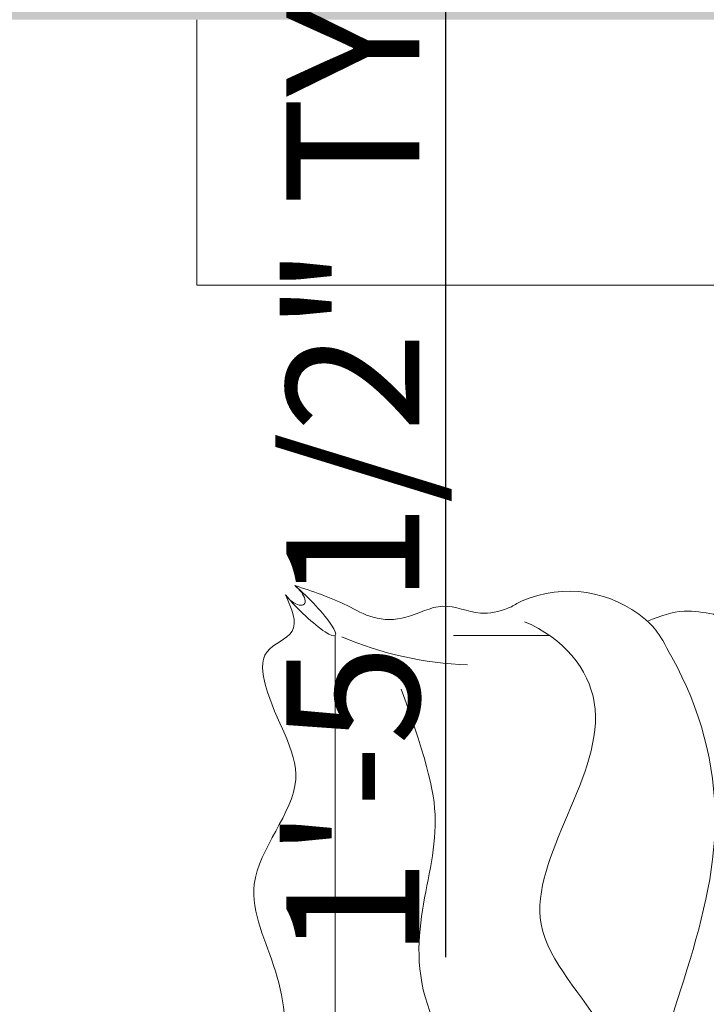
# Model space of a CAD drawing. Units: inches. Extents: x 2083 to 3317, y 1141 to 2115.
# Tile 122 of 256: x 3006 to 3068, y 1327 to 1416. Entities that reach past the tile are written whole.
import ezdxf

# ---------------------------------------------------------------- set-up
doc = ezdxf.new("R2010")
doc.units = ezdxf.units.IN
for name, color, linetype, lineweight in [('A-ANNO-DIMS', 2, 'Continuous', 18), ('A-FLOR-CASE', 8, 'Continuous', 18), ('A-FURN', 8, 'Continuous', 18), ('www.cadblocksfree.com', 7, 'Continuous', 9)]:
    doc.layers.add(name, color=color, linetype=linetype, lineweight=lineweight)
doc.layers.add('A-WALL-PATT', color=251, linetype='Continuous', lineweight=13, true_color=0x636466)
doc.styles.get("Standard").update_dxf_attribs({"font": 'arial.ttf'})
doc.dimstyles.new('ISO-25', dxfattribs={"dimtxt": 12, "dimasz": 12, "dimexe": 1.25, "dimexo": 0.625, "dimtad": 1, "dimlunit": 3, "dimtxsty": 'Standard', "dimcen": 2.5, "dimadec": 0, "dimazin": 0, "dimtfac": 1, "dimtmove": 0, "dimatfit": 3, "dimfxl": 1, "dimarcsym": 0})

# ---------------------------------------------------------------- blocks, each defined once
blk = doc.blocks.new('bed')
at = {"layer": 'www.cadblocksfree.com', "ltscale": 0.2}
for p, q in [((3363.387, 1412.3), (3363.387, 1402.937)), ((3363.387, 1391.414), (3426.379, 1391.414))]:
    blk.add_line(p, q, dxfattribs=at)
for centre, radius, start, end in [((3370.55, 1414.186), 11.465, 139.46484, 203.37116), ((3367.278, 1412.869), 7.939, 204.0179, 212.61896), ((3331.909, 1405.558), 34.378, 336.84952, 357.90025)]:
    blk.add_arc(centre, radius, start, end, dxfattribs=at)
at = {"layer": 'www.cadblocksfree.com', "ltscale": 0.2, "extrusion": (0, 0, -1)}
for centre, major_axis, ratio, start_param, end_param in [((3360.344, 1388.371), (3.043, 3.043), 0.168252, 4.250342, 8.316029), ((3359.289, 1387.316), (1.055, 1.055), 0.453532, 4.422107, 8.144264)]:
    blk.add_ellipse(centre, major_axis=major_axis, ratio=ratio, start_param=start_param, end_param=end_param, dxfattribs=at)
at = {"layer": 'www.cadblocksfree.com', "ltscale": 0.2}
for points, knots in [([(3365.512, 1424.213), (3370.519, 1427.004), (3381.149, 1429.825), (3396.214, 1425.866), (3410.541, 1420.654), (3420.273, 1432.695), (3425.882, 1426.771), (3428.534, 1423.97)], [0.099185, 0.099185, 0.099185, 0.099185, 0.523647, 0.927087, 1.289918, 1.564439, 1.810555, 1.810555, 1.810555, 1.810555]), ([(3361.336, 1428.309), (3361.334, 1428.297), (3361.16, 1427.338), (3360.778, 1425.173), (3361.469, 1423.14), (3362.014, 1421.845)], [0.3128349, 0.3128349, 0.3128349, 0.3128349, 0.313751, 0.386958, 0.4759027, 0.4759027, 0.4759027, 0.4759027]), ([(3362.057, 1409.866), (3363.638, 1413.65), (3372.978, 1421.337), (3389.682, 1406.045), (3402.396, 1419.984), (3416.037, 1420.167), (3423.233, 1415.231), (3427.827, 1408.899)], [0.029901, 0.029901, 0.029901, 0.029901, 0.276967, 0.797115, 1.093669, 1.464666, 1.788489, 1.788489, 1.788489, 1.788489]), ([(3358.529, 1387.473), (3359.098, 1389.205), (3359.955, 1391.816), (3361.924, 1395.149), (3361.896, 1398.555), (3359.883, 1401.841), (3361.557, 1405.208), (3361.034, 1407.507), (3360.643, 1408.467), (3360.591, 1408.59)], [0, 0, 0, 0, 0.138875, 0.2092702, 0.2901949, 0.3858479, 0.4804923, 0.5489252, 0.5590752, 0.5590752, 0.5590752, 0.5590752]), ([(3368.632, 1397.839), (3375.978, 1400.489), (3385.349, 1402.757), (3397.531, 1395.273), (3413.593, 1410.377), (3407.806, 1395.019), (3420.759, 1398.2)], [0.029901, 0.029901, 0.029901, 0.029901, 0.276967, 0.797115, 1.093669, 1.16836, 1.16836, 1.16836, 1.16836]), ([(3430.32, 1386.556), (3427.327, 1387.653), (3422.148, 1389.55), (3414.529, 1384.137), (3405.607, 1387.046), (3396.29, 1386.314), (3386.838, 1381.282), (3377.742, 1390.272), (3370.778, 1384.799), (3364.626, 1383.966), (3363.275, 1388.265), (3360.778, 1387.151), (3359.446, 1386.556)], [0, 0, 0, 0, 8.93042, 15.449194, 25.485629, 34.878505, 43.598887, 54.554403, 64.16647, 67.461673, 70.610457, 74.213583, 74.213583, 74.213583, 74.213583])]:
    blk.add_open_spline(points, degree=3, knots=knots, dxfattribs=at)
for points in [[(3361.235, 1424.042), (3361.236, 1424.042), (3361.237, 1424.043), (3361.239, 1424.043)], [(3361.837, 1421.637), (3362.352, 1422.25), (3362.867, 1422.863), (3365.512, 1424.213)]]:
    blk.add_open_spline(points, degree=3, dxfattribs=at)
blk = doc.blocks.new('CASEWORK-96X24')
for q in [(0, 0), (24, 96)]:
    blk.add_line((0, 96), q)
blk = doc.blocks.new('*D19')
at = {"layer": 'A-ANNO-DIMS', "color": 0, "lineweight": -2, "transparency": 16777216}
for p, q in [((3044.457, 1486.497), (3044.457, 1498.497)), ((3041.693, 1474.497), (3045.707, 1474.497)), ((3044.457, 1474.497), (3044.457, 1456.781)), ((3041.693, 1456.781), (3045.707, 1456.781)), ((3044.457, 1444.781), (3044.457, 1331.553))]:
    blk.add_line(p, q, dxfattribs=at)
at = {"layer": 'A-ANNO-DIMS', "color": 0, "transparency": 16777216}
for points in [[(3042.457, 1486.497), (3046.457, 1486.497), (3044.457, 1474.497)], [(3042.457, 1444.781), (3046.457, 1444.781), (3044.457, 1456.781)]]:
    blk.add_solid(points, dxfattribs=at)
at = {"layer": 'Defpoints', "color": 0, "transparency": 16777216}
for p in [(3041.068, 1474.497), (3041.068, 1456.781), (3044.457, 1456.781)]:
    blk.add_point(p, dxfattribs=at)
at = {"layer": 'A-ANNO-DIMS', "color": 0, "transparency": 16777216, "insert": (3037.627, 1382.167), "char_height": 12, "attachment_point": 5, "rotation": 90}
blk.add_mtext('1\'-5 1/2" TYP.', dxfattribs=at)

msp = doc.modelspace()

# ---------------------------------------------------------------- hatches: boundary and pattern name
at = {"layer": 'A-WALL-PATT'}
h = msp.add_hatch(color=256, dxfattribs=at)
h.dxf.hatch_style = 1
h.paths.add_polyline_path([(3126.96, 2020.761), (2748.96, 2020.761), (2604.96, 2020.761), (2226.96, 2020.761), (2226.96, 1702.761), (2466.96, 1702.761), (2466.96, 1582.761), (2418.96, 1582.761), (2418.96, 1477.761), (2226.96, 1477.761), (2226.96, 1263.261), (2544.96, 1263.261), (2544.96, 1411.761), (2604.96, 1411.761), (2685.96, 1411.761), (2685.96, 1420.761), (2604.96, 1420.761), (2604.96, 1573.761), (2604.96, 1702.761), (2604.96, 2011.761), (2748.96, 2011.761), (2748.96, 1702.761), (2862.96, 1702.761), (2862.96, 1621.761), (2871.96, 1621.761), (2871.96, 1702.761), (2883.96, 1702.761), (2883.96, 1706.939, -0.026459), (2883.96, 1711.761), (2757.96, 1711.761), (2757.96, 1807.761), (2787.96, 1807.761), (2787.96, 1812.261), (2757.96, 1812.261), (2757.96, 2011.761), (2877.96, 2011.761), (2877.96, 1812.261), (2847.96, 1812.261), (2847.96, 1807.761), (2889.836, 1807.761), (2889.836, 1812.261), (2882.46, 1812.261), (2882.46, 2011.761), (3117.96, 2011.761), (3117.96, 1812.261), (2937.836, 1812.261), (2937.836, 1807.761), (2995.71, 1807.761), (2995.71, 1796.118), (3000.21, 1796.118), (3000.21, 1807.761), (3117.96, 1807.761), (3117.96, 1711.761), (3000.21, 1711.761), (3000.21, 1760.118), (2998.573, 1760.118, -0.020711), (2995.71, 1760.118), (2995.71, 1711.761), (2931.96, 1711.761), (2931.96, 1702.761), (3126.96, 1702.761)])
h.paths.add_polyline_path([(2471.46, 2011.761), (2471.46, 1810.011), (2462.717, 1810.011), (2462.717, 1805.511), (2505.96, 1805.511), (2505.96, 1810.011), (2475.96, 1810.011), (2475.96, 2011.761), (2595.96, 2011.761), (2595.96, 1810.011), (2565.96, 1810.011), (2565.96, 1805.511), (2595.96, 1805.511), (2595.96, 1711.761), (2235.96, 1711.761), (2235.96, 1805.511), (2353.71, 1805.511), (2353.71, 1796.054), (2358.21, 1796.054), (2358.21, 1805.511), (2414.717, 1805.511), (2414.717, 1810.011), (2235.96, 1810.011), (2235.96, 2011.761)], flags=16)
h.paths.add_polyline_path([(2270.205, 1994.61), (2270.205, 1970.61), (2246.205, 1970.61), (2246.205, 1994.61)], flags=0)
edge = h.paths.add_edge_path(flags=0)
edge.add_ellipse((2332.027, 1899.798), major_axis=(-3.043, 3.043), ratio=0.168252, start_angle=-161.33217, end_angle=-156.30711, ccw=False)
edge.add_ellipse((2333.082, 1898.744), major_axis=(-1.055, 1.055), ratio=0.453532, start_angle=-123.37102, end_angle=-94.15911)
edge = h.paths.add_edge_path(flags=0)
edge.add_ellipse((2332.027, 1968.876), major_axis=(3.043, 3.043), ratio=0.168252, start_angle=18.66783, end_angle=23.69289)
edge.add_spline(control_points=[(2332.926, 1970.691), (2332.227, 1970.336), (2330.894, 1969.659), (2328.413, 1970.932), (2327.204, 1967.749), (2324.71, 1969.956), (2322.533, 1967.012), (2320.013, 1971.296), (2317.68, 1968.158), (2316.041, 1967.102), (2315.427, 1966.81)], knot_values=[0, 0, 0, 0, 2.267059, 4.324559, 6.685584, 8.878641, 11.121502, 14.300359, 17.755284, 19.732645, 19.732645, 19.732645, 19.732645], degree=3, periodic=0)
edge.add_ellipse((2332.027, 1968.876), major_axis=(3.043, 3.043), ratio=0.168252, start_angle=18.66783, end_angle=23.69289, ccw=False)
edge.add_ellipse((2333.082, 1969.931), major_axis=(1.055, 1.055), ratio=0.453532, start_angle=56.62898, end_angle=85.84089, ccw=False)
edge = h.paths.add_edge_path(flags=0)
edge.add_spline(control_points=[(2296.428, 1967.988), (2293.628, 1965.336), (2287.704, 1959.727), (2299.744, 1949.996), (2294.533, 1935.669), (2290.573, 1920.604), (2293.394, 1909.974), (2296.185, 1904.967)], knot_values=[0.099185, 0.099185, 0.099185, 0.099185, 0.345301, 0.619822, 0.982653, 1.386093, 1.810555, 1.810555, 1.810555, 1.810555], degree=3, periodic=0)
edge.add_spline(control_points=[(2296.185, 1904.967), (2297.384, 1902.619), (2298.001, 1901.949), (2298.553, 1901.468)], knot_values=[0.006246, 0.006246, 0.006246, 0.006246, 0.055476, 0.055476, 0.055476, 0.055476], degree=3, periodic=0)
edge.add_spline(control_points=[(2298.553, 1901.468), (2297.259, 1900.923), (2295.225, 1900.232), (2293.06, 1900.614), (2292.101, 1900.788), (2292.09, 1900.791)], knot_values=[0.312835, 0.312835, 0.312835, 0.312835, 0.40178, 0.474987, 0.475903, 0.475903, 0.475903, 0.475903], degree=3, periodic=0)
edge.add_arc((2292.794, 1904.664), 3.937, 215.4209, 259.69818, ccw=False)
edge.add_spline(control_points=[(2289.585, 1902.382), (2289.477, 1902.535), (2289.368, 1902.688), (2289.261, 1902.841)], knot_values=[0.102872, 0.102872, 0.102872, 0.102872, 0.116896, 0.116896, 0.116896, 0.116896], degree=3, periodic=0)
edge.add_spline(control_points=[(2289.261, 1902.841), (2288.687, 1902.55), (2287.64, 1902.02), (2285.881, 1901.874), (2283.853, 1901.504), (2281.72, 1899.711), (2278.467, 1899.493), (2276.157, 1901.883), (2272.259, 1899.804), (2267.778, 1901.843), (2262.244, 1900.184), (2257.415, 1901.782), (2254.318, 1900.726), (2253.178, 1900.337)], knot_values=[0, 0, 0, 0, 1.907977, 3.477176, 5.261074, 7.972851, 11.680248, 13.717921, 16.939592, 22.789562, 27.502503, 33.595215, 37.145618, 37.145618, 37.145618, 37.145618], degree=3, periodic=0)
edge.add_line((2253.178, 1900.337), (2250.244, 1902.841))
edge.add_line((2250.244, 1902.841), (2250.244, 1965.833))
edge.add_line((2250.244, 1965.833), (2253.178, 1968.337))
edge.add_spline(control_points=[(2253.178, 1968.337), (2254.318, 1967.948), (2257.415, 1966.892), (2262.244, 1968.49), (2267.778, 1966.831), (2271.527, 1968.537), (2273.876, 1967.828), (2274.207, 1967.728)], knot_values=[0, 0, 0, 0, 0.09018, 0.244935, 0.364644, 0.513233, 0.537855, 0.537855, 0.537855, 0.537855], degree=3, periodic=0)
edge.add_arc((2274.353, 1963.793), 3.937, 72.05113, 92.12795, ccw=False)
edge.add_arc((2281.297, 1985.23), 18.596, 252.05113, 288.56572)
edge.add_arc((2292.317, 1956.029), 12.646, 71.02679, 113.77822, ccw=False)
edge = h.paths.add_edge_path(flags=0)
edge.add_spline(control_points=[(2274.899, 1951.856), (2275.066, 1951.617), (2275.233, 1951.377), (2275.398, 1951.136)], knot_values=[1.409916, 1.409916, 1.409916, 1.409916, 1.43159, 1.43159, 1.43159, 1.43159], degree=3, periodic=0)
edge.add_spline(control_points=[(2275.398, 1951.136), (2275.792, 1950.562), (2276.179, 1949.984), (2276.546, 1949.397)], knot_values=[1.358238, 1.358238, 1.358238, 1.358238, 1.409916, 1.409916, 1.409916, 1.409916], degree=3, periodic=0)
edge.add_line((2276.546, 1949.397), (2277.437, 1947.862))
edge.add_spline(control_points=[(2277.437, 1947.862), (2276.304, 1945.673), (2274.64, 1942.427), (2274.632, 1938.094), (2272.799, 1930.852), (2274.356, 1943.897), (2275.948, 1947.923), (2276.546, 1949.397)], knot_values=[0.005632, 0.005632, 0.005632, 0.005632, 0.186014, 0.266002, 0.357087, 0.59639, 0.739732, 0.739732, 0.739732, 0.739732], degree=3, periodic=0)
edge.add_spline(control_points=[(2276.546, 1949.397), (2276.179, 1949.984), (2275.792, 1950.562), (2275.398, 1951.136)], knot_values=[1.358238, 1.358238, 1.358238, 1.358238, 1.409916, 1.409916, 1.409916, 1.409916], degree=3, periodic=0)
edge.add_spline(control_points=[(2275.398, 1951.136), (2274.943, 1950.08), (2274.208, 1948.025), (2273.935, 1944.851), (2272.469, 1937.627), (2273.466, 1945.696), (2274.701, 1951.059), (2274.899, 1951.856)], knot_values=[0.104364, 0.104364, 0.104364, 0.104364, 0.189636, 0.269624, 0.36071, 0.600013, 0.644622, 0.644622, 0.644622, 0.644622], degree=3, periodic=0)
h.paths.add_polyline_path([(2269.168, 1963.128, -0.357527), (2268.171, 1960.976, -0.092561), (2268.171, 1939.436, -0.357527), (2269.168, 1937.285, -0.357527), (2267.016, 1938.282, -0.164785), (2254.686, 1938.282, -0.357527), (2252.534, 1937.285, -0.357527), (2253.531, 1939.436, -0.092561), (2253.531, 1960.976, -0.357527), (2252.534, 1963.128, -0.357527), (2254.686, 1962.131, -0.164785), (2267.016, 1962.131, -0.357527)], flags=0)
h.paths.add_polyline_path([(2248.874, 1967.802), (2248.874, 1957.028), (2249.458, 1957.028), (2249.458, 1911.647), (2248.874, 1911.647), (2248.874, 1900.873), (2246.512, 1900.873, 0.197327), (2244.15, 1902.457), (2244.15, 1966.218, 0.197327), (2246.512, 1967.802)], flags=0)
h.paths.add_polyline_path([(2269.168, 1931.389, -0.357527), (2268.171, 1929.238, -0.092561), (2268.171, 1907.698, -0.357527), (2269.168, 1905.547, -0.357527), (2267.016, 1906.544, -0.164785), (2254.686, 1906.544, -0.357527), (2252.534, 1905.547, -0.357527), (2253.531, 1907.698, -0.092561), (2253.531, 1929.238, -0.357527), (2252.534, 1931.389, -0.357527), (2254.686, 1930.392, -0.164785), (2267.016, 1930.392, -0.357527)], flags=0)
edge = h.paths.add_edge_path(flags=0)
edge.add_spline(control_points=[(2276.197, 1906.724), (2276.168, 1909.029), (2276.114, 1913.372), (2270.598, 1924.925), (2273.905, 1919.013), (2275.922, 1916.262), (2275.475, 1912.402), (2277.258, 1910.381), (2276.696, 1908.225), (2276.646, 1906.813), (2276.618, 1906.008)], knot_values=[0, 0, 0, 0, 8.61026, 16.221274, 18.843057, 23.804898, 27.440828, 29.356102, 31.203478, 33.650687, 33.650687, 33.650687, 33.650687], degree=3, periodic=0)
edge.add_spline(control_points=[(2276.618, 1906.008), (2276.623, 1905.624), (2276.498, 1904.629), (2275.442, 1903.855), (2274.937, 1903.08), (2274.859, 1902.841)], knot_values=[0.156488, 0.156488, 0.156488, 0.156488, 0.184398, 0.231376, 0.250598, 0.250598, 0.250598, 0.250598], degree=3, periodic=0)
edge.add_line((2274.859, 1902.841), (2276.506, 1902.841))
edge.add_spline(control_points=[(2276.506, 1902.841), (2276.788, 1903.085), (2277.665, 1904.125), (2278.25, 1904.341), (2277.654, 1908.527), (2278.156, 1906.228), (2278.1, 1905.286), (2278.847, 1904.069), (2277.857, 1903.415), (2277.874, 1902.991), (2277.904, 1902.841)], knot_values=[0.059574, 0.059574, 0.059574, 0.059574, 0.080753, 0.103741, 0.16972, 0.176036, 0.207137, 0.240474, 0.262341, 0.27366, 0.27366, 0.27366, 0.27366], degree=3, periodic=0)
edge.add_line((2277.904, 1902.841), (2280.03, 1902.841))
edge.add_spline(control_points=[(2280.03, 1902.841), (2279.888, 1903.088), (2279.499, 1903.982), (2280.152, 1905.939), (2278.104, 1909.658), (2279.762, 1907.185), (2280.328, 1904.875), (2280.485, 1903.49), (2281.463, 1903.249), (2281.758, 1902.936), (2281.834, 1902.841)], knot_values=[0.013856, 0.013856, 0.013856, 0.013856, 0.034874, 0.088867, 0.107879, 0.126738, 0.158714, 0.193757, 0.217487, 0.226722, 0.226722, 0.226722, 0.226722], degree=3, periodic=0)
edge.add_spline(control_points=[(2281.834, 1902.841), (2281.788, 1902.827), (2281.647, 1902.783), (2281.396, 1902.859), (2281.088, 1902.985), (2280.721, 1903.061), (2280.333, 1903.026), (2280.125, 1902.899), (2280.03, 1902.841)], knot_values=[0, 0, 0, 0, 0.14413, 0.435517, 0.749276, 1.153046, 1.548371, 1.878348, 1.878348, 1.878348, 1.878348], degree=3, periodic=0)
edge.add_line((2280.03, 1902.841), (2277.904, 1902.841))
edge.add_spline(control_points=[(2277.904, 1902.841), (2277.893, 1902.796), (2277.865, 1902.68), (2277.607, 1902.687), (2277.274, 1902.801), (2276.838, 1902.62), (2276.584, 1902.789), (2276.506, 1902.841)], knot_values=[0, 0, 0, 0, 0.127189, 0.326199, 0.628009, 1.24357, 1.515331, 1.515331, 1.515331, 1.515331], degree=3, periodic=0)
edge.add_line((2276.506, 1902.841), (2274.859, 1902.841))
edge.add_spline(control_points=[(2274.859, 1902.841), (2274.814, 1902.899), (2274.725, 1903.013), (2274.493, 1903.119), (2274.244, 1902.961), (2273.937, 1903.185), (2273.614, 1902.983), (2273.408, 1902.883), (2273.322, 1902.841)], knot_values=[0, 0, 0, 0, 0.21843, 0.436957, 0.687977, 0.990379, 1.398396, 1.69185, 1.69185, 1.69185, 1.69185], degree=3, periodic=0)
edge.add_spline(control_points=[(2273.322, 1902.841), (2273.617, 1903.446), (2274.274, 1904.538), (2276.027, 1904.574), (2276.207, 1906.584), (2276.197, 1906.724)], knot_values=[0.012227, 0.012227, 0.012227, 0.012227, 0.059472, 0.106218, 0.134458, 0.134458, 0.134458, 0.134458], degree=3, periodic=0)
h.paths.add_polyline_path([(2270.776, 1897.79), (2270.776, 1873.79), (2246.776, 1873.79), (2246.776, 1897.79)], flags=0)
h.paths.add_polyline_path([(2353.71, 1760.005), (2353.71, 1760.054), (2358.21, 1760.054, -0.033729)], flags=0)
h.paths.add_polyline_path([(2321.819, 1737.529), (2341.995, 1737.529, -0.414214), (2343.203, 1736.321), (2343.203, 1721.021, -0.414214), (2341.995, 1719.813), (2321.819, 1719.813, -0.414214), (2320.611, 1721.021), (2320.611, 1736.321, -0.414214)], flags=0)
h.paths.add_polyline_path([(2324.235, 1736.321), (2339.579, 1736.321, -0.414214), (2341.995, 1733.905), (2341.995, 1725.45, -0.414214), (2339.579, 1723.034), (2333.681, 1723.034), (2333.845, 1722.045, -0.870646), (2335.425, 1721.826, -0.767327), (2333.923, 1721.423), (2331.291, 1721.423, -0.767327), (2329.788, 1721.826, -0.870646), (2331.368, 1722.045), (2331.533, 1723.034), (2324.235, 1723.034, -0.414214), (2321.819, 1725.45), (2321.819, 1733.905, -0.414214)], flags=0)
h.paths.add_polyline_path([(2570.484, 1928.615), (2589.684, 1928.615), (2590.169, 1928.615), (2590.169, 1904.993), (2570.484, 1904.993)], flags=0)
h.paths.add_polyline_path([(2574.447, 1927.264, -1), (2572.829, 1927.264, -1)], flags=0)
h.paths.add_polyline_path([(2573.09, 1926.941), (2573.925, 1927.776), (2574.148, 1927.553), (2573.313, 1926.718)], flags=0)
h.paths.add_polyline_path([(2578.779, 1919.73, -1), (2571.592, 1919.73, -1)], flags=0)
h.paths.add_polyline_path([(2578.385, 1919.73, -1), (2571.985, 1919.73, -1)], flags=0)
h.paths.add_polyline_path([(2331.596, 1729.476, -1), (2333.618, 1729.476, -1)], flags=0)
h.paths.add_polyline_path([(2578.034, 1927.264, -1), (2576.416, 1927.264, -1)], flags=0)
h.paths.add_polyline_path([(2576.689, 1927.531), (2576.912, 1927.754), (2577.747, 1926.919), (2577.524, 1926.696)], flags=0)
h.paths.add_polyline_path([(2578.139, 1909.86, -1), (2572.232, 1909.86, -1)], flags=0)
h.paths.add_polyline_path([(2577.745, 1909.86, -1), (2572.625, 1909.86, -1)], flags=0)
h.paths.add_polyline_path([(2583.798, 1927.264, -1), (2582.179, 1927.264, -1)], flags=0)
h.paths.add_polyline_path([(2582.719, 1927.754), (2583.554, 1926.919), (2583.331, 1926.696), (2582.496, 1927.531)], flags=0)
h.paths.add_polyline_path([(2582.496, 1927.531), (2582.719, 1927.754), (2583.554, 1926.919), (2583.331, 1926.696)], flags=0)
h.paths.add_polyline_path([(2587.739, 1920.53, -1), (2581.832, 1920.53, -1)], flags=0)
h.paths.add_polyline_path([(2587.345, 1920.53, -1), (2582.225, 1920.53, -1)], flags=0)
h.paths.add_polyline_path([(2587.385, 1927.264, -1), (2585.766, 1927.264, -1)], flags=0)
h.paths.add_polyline_path([(2586.082, 1926.98), (2586.917, 1927.815), (2587.14, 1927.593), (2586.305, 1926.758)], flags=0)
h.paths.add_polyline_path([(2588.379, 1910.66, -1), (2581.192, 1910.66, -1)], flags=0)
h.paths.add_polyline_path([(2587.985, 1910.66, -1), (2581.585, 1910.66, -1)], flags=0)
h.paths.add_polyline_path([(2417.168, 1729.478), (2437.344, 1729.478, -0.414214), (2438.552, 1728.27), (2438.552, 1712.969, -0.414214), (2437.344, 1711.761), (2417.168, 1711.761, -0.414214), (2415.96, 1712.969), (2415.96, 1728.27, -0.414214)], flags=0)
h.paths.add_polyline_path([(2419.584, 1728.27), (2434.928, 1728.27, -0.414214), (2437.344, 1725.854), (2437.344, 1717.398, -0.414214), (2434.928, 1714.983), (2429.029, 1714.983), (2429.194, 1713.994, -0.870646), (2430.774, 1713.775, -0.767327), (2429.271, 1713.372), (2426.64, 1713.372, -0.767327), (2425.137, 1713.775, -0.870646), (2426.717, 1713.994), (2426.882, 1714.983), (2419.584, 1714.983, -0.414214), (2417.168, 1717.398), (2417.168, 1725.854, -0.414214)], flags=0)
h.paths.add_polyline_path([(2419.584, 1728.27), (2434.928, 1728.27, -0.414214), (2437.344, 1725.854), (2437.344, 1717.398, -0.414214), (2434.928, 1714.983), (2429.029, 1714.983), (2428.358, 1719.009), (2427.553, 1719.009), (2426.882, 1714.983), (2419.584, 1714.983, -0.414214), (2417.168, 1717.398), (2417.168, 1725.854, -0.414214)], flags=0)
h.paths.add_polyline_path([(2426.944, 1721.425, -1), (2428.967, 1721.425, -1)], flags=0)
h.paths.add_polyline_path([(2475.96, 1702.761), (2595.96, 1702.761), (2595.96, 1582.761), (2475.96, 1582.761)], flags=16)
h.paths.add_polyline_path([(2427.96, 1573.761), (2595.96, 1573.761), (2595.96, 1468.761), (2595.96, 1420.761), (2384.46, 1420.761), (2384.46, 1468.761), (2427.96, 1468.761)], flags=16)
h.paths.add_polyline_path([(2379.96, 1468.761), (2379.96, 1420.761), (2235.96, 1420.761), (2235.96, 1468.761)], flags=16)
h.paths.add_polyline_path([(2317.816, 1466.696), (2337.992, 1466.696, -0.414214), (2339.2, 1465.488), (2339.2, 1450.187, -0.414214), (2337.992, 1448.979), (2317.816, 1448.979, -0.414214), (2316.608, 1450.187), (2316.608, 1465.488, -0.414214)], flags=0)
h.paths.add_polyline_path([(2320.232, 1465.488), (2335.576, 1465.488, -0.414214), (2337.992, 1463.072), (2337.992, 1454.616, -0.414214), (2335.576, 1452.2), (2329.677, 1452.2), (2329.842, 1451.212, -0.870646), (2331.422, 1450.992, -0.767327), (2329.92, 1450.59), (2327.288, 1450.59, -0.767327), (2325.785, 1450.992, -0.870646), (2327.365, 1451.212), (2327.53, 1452.2), (2320.232, 1452.2, -0.414214), (2317.816, 1454.616), (2317.816, 1463.072, -0.414214)], flags=0)
h.paths.add_polyline_path([(2320.232, 1465.488), (2335.576, 1465.488, -0.414214), (2337.992, 1463.072), (2337.992, 1454.616, -0.414214), (2335.576, 1452.2), (2329.677, 1452.2), (2329.006, 1456.227), (2328.201, 1456.227), (2327.53, 1452.2), (2320.232, 1452.2, -0.414214), (2317.816, 1454.616), (2317.816, 1463.072, -0.414214)], flags=0)
h.paths.add_polyline_path([(2327.593, 1458.643, -1), (2329.615, 1458.643, -1)], flags=0)
h.paths.add_polyline_path([(2244.412, 1433.34), (2241.921, 1433.34, -0.414214), (2240.018, 1435.244), (2240.018, 1440.953, -0.414211), (2241.921, 1442.856), (2244.412, 1442.856, -1.976472)], flags=0)
h.paths.add_polyline_path([(2245.357, 1434.398, -0.414214), (2245.357, 1441.799, -2.144098)], flags=0)
h.paths.add_polyline_path([(2535.96, 1416.261), (2535.96, 1272.261), (2235.96, 1272.261), (2235.96, 1416.261)], flags=16)
h.paths.add_polyline_path([(2260.12, 1384.293), (2260.12, 1362.039), (2237.865, 1362.039), (2237.865, 1384.293)], flags=0)
edge = h.paths.add_edge_path(flags=0)
edge.add_line((2318.252, 1362.093), (2318.146, 1362.001))
edge.add_ellipse((2317.445, 1360.431), major_axis=(2.822, 2.822), ratio=0.168252, start_angle=18.66783, end_angle=20.94813, ccw=False)
edge.add_ellipse((2318.423, 1361.409), major_axis=(0.978, 0.978), ratio=0.453532, start_angle=56.62898, end_angle=70.2262, ccw=False)
edge = h.paths.add_edge_path(flags=0)
edge.add_line((2319.107, 1295.571), (2319.015, 1295.677))
edge.add_ellipse((2317.445, 1296.378), major_axis=(-2.822, 2.822), ratio=0.168252, start_angle=-161.33217, end_angle=-159.05187, ccw=False)
edge.add_ellipse((2318.423, 1295.4), major_axis=(-0.978, 0.978), ratio=0.453532, start_angle=-123.37102, end_angle=-109.7738)
edge = h.paths.add_edge_path(flags=0)
edge.add_spline(control_points=[(2284.21, 1301.17), (2284.581, 1300.445), (2284.891, 1299.892), (2285.16, 1299.461)], knot_values=[0.039066, 0.039066, 0.039066, 0.039066, 0.055476, 0.055476, 0.055476, 0.055476], degree=3, periodic=0)
edge.add_line((2285.16, 1299.461), (2284.21, 1301.17))
edge = h.paths.add_edge_path(flags=0)
edge.add_line((2280.412, 1297.298), (2283.37, 1297.036))
edge.add_line((2283.37, 1297.036), (2286.406, 1297.926))
edge.add_spline(control_points=[(2286.406, 1297.926), (2285.305, 1297.463), (2284.345, 1297.129), (2283.37, 1297.036)], knot_values=[0.394369, 0.394369, 0.394369, 0.394369, 0.475903, 0.475903, 0.475903, 0.475903], degree=3, periodic=0)
edge.add_spline(control_points=[(2283.37, 1297.036), (2283.281, 1297.028), (2282.316, 1296.957), (2281.313, 1297.134), (2280.423, 1297.296), (2280.412, 1297.298)], knot_values=[0.312835, 0.312835, 0.312835, 0.312835, 0.320246, 0.393453, 0.394369, 0.394369, 0.394369, 0.394369], degree=3, periodic=0)
edge = h.paths.add_edge_path(flags=0)
edge.add_line((2284.436, 1359.607), (2280.446, 1355.328))
edge.add_line((2280.446, 1355.328), (2279.58, 1351.018))
edge.add_line((2279.58, 1351.018), (2282.413, 1346.58))
edge.add_spline(control_points=[(2282.413, 1346.58), (2283.153, 1345.589), (2284.253, 1344.029), (2284.801, 1342.387), (2284.935, 1341.806)], knot_values=[1.240098, 1.240098, 1.240098, 1.240098, 1.332892, 1.382712, 1.382712, 1.382712, 1.382712], degree=3, periodic=0)
edge.add_spline(control_points=[(2284.935, 1341.806), (2285.319, 1340.141), (2285.233, 1338.409), (2284.91, 1336.654)], knot_values=[1.097484, 1.097484, 1.097484, 1.097484, 1.240098, 1.240098, 1.240098, 1.240098], degree=3, periodic=0)
edge.add_spline(control_points=[(2284.91, 1336.654), (2284.587, 1334.899), (2284.027, 1333.12), (2283.463, 1331.361)], knot_values=[0.95487, 0.95487, 0.95487, 0.95487, 1.097484, 1.097484, 1.097484, 1.097484], degree=3, periodic=0)
edge.add_line((2283.463, 1331.361), (2281.89, 1326.153))
edge.add_line((2281.89, 1326.153), (2280.756, 1321.056))
edge.add_line((2280.756, 1321.056), (2280.299, 1316.002))
edge.add_line((2280.299, 1316.002), (2280.716, 1310.95))
edge.add_line((2280.716, 1310.95), (2282.028, 1305.972))
edge.add_line((2282.028, 1305.972), (2284.21, 1301.17))
edge.add_spline(control_points=[(2284.21, 1301.17), (2283.341, 1302.73), (2282.612, 1304.336), (2282.028, 1305.972)], knot_values=[0.099185, 0.099185, 0.099185, 0.099185, 0.241799, 0.241799, 0.241799, 0.241799], degree=3, periodic=0)
edge.add_spline(control_points=[(2282.028, 1305.972), (2281.444, 1307.608), (2281.005, 1309.273), (2280.716, 1310.95)], knot_values=[0.241799, 0.241799, 0.241799, 0.241799, 0.384413, 0.384413, 0.384413, 0.384413], degree=3, periodic=0)
edge.add_spline(control_points=[(2280.716, 1310.95), (2280.433, 1312.588), (2280.289, 1314.277), (2280.299, 1315.962), (2280.299, 1316.002)], knot_values=[0.384413, 0.384413, 0.384413, 0.384413, 0.523647, 0.527028, 0.527028, 0.527028, 0.527028], degree=3, periodic=0)
edge.add_spline(control_points=[(2280.299, 1316.002), (2280.312, 1317.687), (2280.478, 1319.368), (2280.756, 1321.056)], knot_values=[0.527028, 0.527028, 0.527028, 0.527028, 0.669642, 0.669642, 0.669642, 0.669642], degree=3, periodic=0)
edge.add_spline(control_points=[(2280.756, 1321.056), (2281.035, 1322.744), (2281.426, 1324.44), (2281.89, 1326.153)], knot_values=[0.669642, 0.669642, 0.669642, 0.669642, 0.812256, 0.812256, 0.812256, 0.812256], degree=3, periodic=0)
edge.add_spline(control_points=[(2281.89, 1326.153), (2282.264, 1327.533), (2282.788, 1329.262), (2283.353, 1331.018), (2283.463, 1331.361)], knot_values=[0.812256, 0.812256, 0.812256, 0.812256, 0.927087, 0.95487, 0.95487, 0.95487, 0.95487], degree=3, periodic=0)
edge.add_line((2283.463, 1331.361), (2284.91, 1336.654))
edge.add_line((2284.91, 1336.654), (2284.935, 1341.806))
edge.add_line((2284.935, 1341.806), (2282.413, 1346.58))
edge.add_spline(control_points=[(2282.413, 1346.58), (2281.275, 1348.104), (2280.078, 1349.57), (2279.58, 1351.018)], knot_values=[1.382712, 1.382712, 1.382712, 1.382712, 1.525326, 1.525326, 1.525326, 1.525326], degree=3, periodic=0)
edge.add_spline(control_points=[(2279.58, 1351.018), (2279.443, 1351.415), (2279.136, 1352.857), (2279.735, 1354.29), (2280.446, 1355.328)], knot_values=[1.525326, 1.525326, 1.525326, 1.525326, 1.564439, 1.667941, 1.667941, 1.667941, 1.667941], degree=3, periodic=0)
edge.add_spline(control_points=[(2280.446, 1355.328), (2281.426, 1356.758), (2282.931, 1358.183), (2284.436, 1359.607)], knot_values=[1.667941, 1.667941, 1.667941, 1.667941, 1.810555, 1.810555, 1.810555, 1.810555], degree=3, periodic=0)
edge.add_arc((2280.623, 1348.518), 11.726, 71.02679, 113.77822)
edge.add_arc((2270.405, 1375.595), 17.244, 252.05113, 288.56572, ccw=False)
edge.add_arc((2263.966, 1355.718), 3.651, 72.05113, 92.12795)
edge.add_arc((2263.966, 1355.718), 3.651, 92.12795, 177.98513)
edge.add_spline(control_points=[(2260.318, 1355.846), (2260.26, 1354.221), (2260.551, 1350.187), (2262.999, 1346.766), (2264.473, 1344.649)], knot_values=[1.43159, 1.43159, 1.43159, 1.43159, 1.564144, 1.770695, 1.770695, 1.770695, 1.770695], degree=3, periodic=0)
edge.add_line((2264.473, 1344.649), (2264.936, 1343.983))
edge.add_spline(control_points=[(2263.801, 1340.248), (2263.843, 1340.514), (2264.067, 1341.756), (2264.513, 1343.002), (2264.935, 1343.981)], knot_values=[0.53657, 0.53657, 0.53657, 0.53657, 0.559349, 0.644622, 0.644622, 0.644622, 0.644622], degree=3, periodic=0)
edge.add_spline(control_points=[(2264.935, 1343.981), (2265.118, 1343.715), (2265.299, 1343.448), (2265.477, 1343.179)], knot_values=[1.384077, 1.384077, 1.384077, 1.384077, 1.409916, 1.409916, 1.409916, 1.409916], degree=3, periodic=0)
edge.add_spline(control_points=[(2265.477, 1343.179), (2265.655, 1342.911), (2265.829, 1342.641), (2265.999, 1342.369)], knot_values=[1.358238, 1.358238, 1.358238, 1.358238, 1.384077, 1.384077, 1.384077, 1.384077], degree=3, periodic=0)
edge.add_line((2265.999, 1342.369), (2266.826, 1340.946))
edge.add_spline(control_points=[(2266.826, 1340.946), (2268.894, 1337.09), (2271.398, 1325.843), (2270.516, 1310.569), (2275.919, 1301.861), (2277.79, 1299.199)], knot_values=[0.116896, 0.116896, 0.116896, 0.116896, 0.472987, 1.050969, 1.313793, 1.313793, 1.313793, 1.313793], degree=3, periodic=0)
edge.add_spline(control_points=[(2277.79, 1299.199), (2277.839, 1299.128), (2277.889, 1299.057), (2277.94, 1298.987)], knot_values=[0.109884, 0.109884, 0.109884, 0.109884, 0.116896, 0.116896, 0.116896, 0.116896], degree=3, periodic=0)
edge.add_line((2277.94, 1298.987), (2277.789, 1299.199))
edge.add_spline(control_points=[(2277.789, 1299.199), (2277.257, 1298.929), (2276.286, 1298.438), (2275.039, 1298.334), (2274.383, 1298.239), (2274.215, 1298.209)], knot_values=[33.12187, 33.12187, 33.12187, 33.12187, 35.029056, 36.598255, 37.144827, 37.144827, 37.144827, 37.144827], degree=3, periodic=0)
edge.add_line((2274.215, 1298.209), (2273.073, 1297.893))
edge.add_spline(control_points=[(2273.073, 1297.893), (2272.323, 1297.58), (2271.039, 1296.511), (2269.248, 1296.226), (2268.423, 1296.375)], knot_values=[26.532584, 26.532584, 26.532584, 26.532584, 29.198919, 31.839101, 31.839101, 31.839101, 31.839101], degree=3, periodic=0)
edge.add_line((2268.423, 1296.375), (2263.879, 1297.458))
edge.add_spline(control_points=[(2263.879, 1297.458), (2263.556, 1297.359), (2261.86, 1296.839), (2260.239, 1297.282), (2258.933, 1297.516)], knot_values=[15.919551, 15.919551, 15.919551, 15.919551, 16.939592, 21.226067, 21.226067, 21.226067, 21.226067], degree=3, periodic=0)
edge.add_line((2258.933, 1297.516), (2254.055, 1297.329))
edge.add_spline(control_points=[(2254.055, 1297.329), (2253.756, 1297.296), (2252.114, 1297.165), (2250.462, 1297.544), (2249.13, 1297.668)], knot_values=[5.306517, 5.306517, 5.306517, 5.306517, 6.276435, 10.613034, 10.613034, 10.613034, 10.613034], degree=3, periodic=0)
edge.add_line((2249.13, 1297.668), (2244.332, 1296.878))
edge.add_line((2244.332, 1296.878), (2241.611, 1299.199))
edge.add_line((2241.611, 1299.199), (2241.611, 1357.609))
edge.add_line((2241.611, 1357.609), (2244.332, 1359.931))
edge.add_line((2244.332, 1359.931), (2252.729, 1359.543))
edge.add_spline(control_points=[(2252.729, 1359.543), (2252.871, 1359.546), (2253.306, 1359.548), (2253.74, 1359.514), (2254.032, 1359.482)], knot_values=[0.233291, 0.233291, 0.233291, 0.233291, 0.244935, 0.268927, 0.268927, 0.268927, 0.268927], degree=3, periodic=0)
edge.add_line((2254.032, 1359.482), (2259.587, 1359.416))
edge.add_spline(control_points=[(2259.587, 1359.416), (2260.677, 1359.629), (2262.073, 1359.897), (2263.524, 1359.459), (2263.83, 1359.366)], knot_values=[0.422516, 0.422516, 0.422516, 0.422516, 0.513233, 0.537855, 0.537855, 0.537855, 0.537855], degree=3, periodic=0)
edge.add_arc((2263.966, 1355.718), 3.651, 72.05113, 92.12795, ccw=False)
edge.add_arc((2270.405, 1375.595), 17.244, 252.05113, 288.56572)
edge.add_arc((2280.623, 1348.518), 11.726, 71.02679, 113.77822, ccw=False)
h.paths.add_polyline_path([(2240.341, 1359.435), (2240.341, 1349.444), (2240.882, 1349.444), (2240.882, 1307.365), (2240.341, 1307.365), (2240.341, 1297.374), (2238.15, 1297.374, 0.197327), (2235.96, 1298.843), (2235.96, 1357.966, 0.197327), (2238.15, 1359.435)], flags=0)
h.paths.add_polyline_path([(2259.158, 1355.101, -0.357527), (2258.233, 1353.106, -0.092561), (2258.233, 1333.133, -0.357527), (2259.158, 1331.138, -0.357527), (2257.163, 1332.062, -0.164785), (2245.729, 1332.062, -0.357527), (2243.735, 1331.138, -0.357527), (2244.659, 1333.133, -0.092561), (2244.659, 1353.106, -0.357527), (2243.735, 1355.101, -0.357527), (2245.729, 1354.176, -0.164785), (2257.163, 1354.176, -0.357527)], flags=0)
edge = h.paths.add_edge_path(flags=0)
edge.add_line((2265.999, 1342.369), (2266.826, 1340.946))
edge.add_line((2266.826, 1340.946), (2265.308, 1337.814))
edge.add_line((2265.308, 1337.814), (2264.358, 1334.653))
edge.add_line((2264.358, 1334.653), (2264.262, 1333.8))
edge.add_spline(control_points=[(2264.262, 1333.8), (2264.208, 1333.187), (2264.162, 1332.366), (2264.007, 1331.414), (2263.969, 1331.202)], knot_values=[0.464444, 0.464444, 0.464444, 0.464444, 0.516691, 0.531608, 0.531608, 0.531608, 0.531608], degree=3, periodic=0)
edge.add_spline(control_points=[(2263.969, 1331.202), (2263.775, 1330.119), (2263.424, 1328.791), (2263.257, 1328.531), (2263.234, 1328.515)], knot_values=[0.372682, 0.372682, 0.372682, 0.372682, 0.44885, 0.464444, 0.464444, 0.464444, 0.464444], degree=3, periodic=0)
edge.add_spline(control_points=[(2263.234, 1328.515), (2263.096, 1328.42), (2263.131, 1329.301), (2263.275, 1330.616)], knot_values=[0.280919, 0.280919, 0.280919, 0.280919, 0.372682, 0.372682, 0.372682, 0.372682], degree=3, periodic=0)
edge.add_spline(control_points=[(2263.275, 1330.616), (2263.419, 1331.93), (2263.672, 1333.677), (2263.97, 1335.315)], knot_values=[0.189157, 0.189157, 0.189157, 0.189157, 0.280919, 0.280919, 0.280919, 0.280919], degree=3, periodic=0)
edge.add_spline(control_points=[(2263.97, 1335.315), (2264.1, 1336.032), (2264.419, 1337.622), (2264.755, 1338.864), (2264.947, 1339.491)], knot_values=[0.097394, 0.097394, 0.097394, 0.097394, 0.137578, 0.189157, 0.189157, 0.189157, 0.189157], degree=3, periodic=0)
edge.add_spline(control_points=[(2264.947, 1339.491), (2265.29, 1340.606), (2265.644, 1341.494), (2265.999, 1342.369)], knot_values=[0.005632, 0.005632, 0.005632, 0.005632, 0.097394, 0.097394, 0.097394, 0.097394], degree=3, periodic=0)
h.paths.add_polyline_path([(2259.158, 1325.671, -0.357527), (2258.233, 1323.676, -0.092561), (2258.233, 1303.703, -0.357527), (2259.158, 1301.708, -0.357527), (2257.163, 1302.633, -0.164785), (2245.729, 1302.633, -0.357527), (2243.735, 1301.708, -0.357527), (2244.659, 1303.703, -0.092561), (2244.659, 1323.676, -0.357527), (2243.735, 1325.671, -0.357527), (2245.729, 1324.747, -0.164785), (2257.163, 1324.747, -0.357527)], flags=0)
edge = h.paths.add_edge_path(flags=0)
edge.add_spline(control_points=[(2261.709, 1317.311), (2261.679, 1317.418), (2261.762, 1317.389), (2262.491, 1316.09), (2262.962, 1315.301)], knot_values=[14.955861, 14.955861, 14.955861, 14.955861, 16.221274, 18.694826, 18.694826, 18.694826, 18.694826], degree=3, periodic=0)
edge.add_spline(control_points=[(2262.962, 1315.301), (2262.99, 1315.254), (2263.702, 1314.067), (2264.349, 1313.127), (2264.73, 1312.164)], knot_values=[18.694826, 18.694826, 18.694826, 18.694826, 18.843057, 22.433791, 22.433791, 22.433791, 22.433791], degree=3, periodic=0)
edge.add_spline(control_points=[(2264.73, 1312.164), (2264.876, 1311.796), (2265.177, 1310.77), (2265.143, 1309.559), (2265.248, 1308.824)], knot_values=[22.433791, 22.433791, 22.433791, 22.433791, 23.804898, 26.172756, 26.172756, 26.172756, 26.172756], degree=3, periodic=0)
edge.add_line((2265.248, 1308.824), (2265.851, 1307.172))
edge.add_spline(control_points=[(2265.851, 1307.172), (2266.065, 1306.822), (2266.384, 1306.332), (2266.424, 1305.781), (2266.42, 1305.611)], knot_values=[28.062562, 28.062562, 28.062562, 28.062562, 29.356102, 29.911721, 29.911721, 29.911721, 29.911721], degree=3, periodic=0)
edge.add_spline(control_points=[(2266.42, 1305.611), (2266.416, 1305.433), (2266.394, 1305.25), (2266.365, 1305.066)], knot_values=[29.911721, 29.911721, 29.911721, 29.911721, 30.497837, 30.497837, 30.497837, 30.497837], degree=3, periodic=0)
edge.add_line((2266.365, 1305.066), (2266.066, 1302.136))
edge.add_spline(control_points=[(2266.066, 1302.136), (2266.071, 1301.78), (2265.998, 1301.2), (2265.663, 1300.759), (2265.509, 1300.586)], knot_values=[0.156488, 0.156488, 0.156488, 0.156488, 0.184398, 0.203543, 0.203543, 0.203543, 0.203543], degree=3, periodic=0)
edge.add_line((2265.509, 1300.586), (2264.435, 1299.199))
edge.add_line((2264.435, 1299.199), (2265.962, 1299.199))
edge.add_line((2265.962, 1299.199), (2267.336, 1301.175))
edge.add_line((2267.336, 1301.175), (2267.312, 1301.986))
edge.add_spline(control_points=[(2267.312, 1301.986), (2267.261, 1302.862), (2267.16, 1303.737), (2267.271, 1303.326)], knot_values=[0.126229, 0.126229, 0.126229, 0.126229, 0.166617, 0.166617, 0.166617, 0.166617], degree=3, periodic=0)
edge.add_spline(control_points=[(2267.271, 1303.326), (2267.28, 1303.294), (2267.31, 1303.175), (2267.373, 1302.884), (2267.406, 1302.683), (2267.418, 1302.601)], knot_values=[0.166617, 0.166617, 0.166617, 0.166617, 0.16972, 0.176036, 0.180765, 0.180765, 0.180765, 0.180765], degree=3, periodic=0)
edge.add_spline(control_points=[(2267.744, 1300.988), (2267.688, 1301.151), (2267.481, 1301.657), (2267.484, 1302.145), (2267.418, 1302.601)], knot_values=[0.180765, 0.180765, 0.180765, 0.180765, 0.193767, 0.220139, 0.220139, 0.220139, 0.220139], degree=3, periodic=0)
edge.add_line((2267.418, 1302.601), (2267.744, 1300.988))
edge.add_spline(control_points=[(2267.744, 1300.988), (2267.832, 1300.732), (2267.932, 1300.31), (2267.555, 1299.975), (2267.429, 1299.829)], knot_values=[0.220139, 0.220139, 0.220139, 0.220139, 0.240474, 0.25489, 0.25489, 0.25489, 0.25489], degree=3, periodic=0)
edge.add_line((2267.429, 1299.829), (2267.258, 1299.199))
edge.add_line((2267.258, 1299.199), (2269.23, 1299.199))
edge.add_spline(control_points=[(2269.23, 1299.199), (2269.099, 1299.429), (2268.843, 1300.016), (2269.012, 1300.916), (2268.947, 1301.661)], knot_values=[0.013856, 0.013856, 0.013856, 0.013856, 0.034874, 0.067073, 0.067073, 0.067073, 0.067073], degree=3, periodic=0)
edge.add_line((2268.947, 1301.661), (2268.432, 1303.603))
edge.add_spline(control_points=[(2268.432, 1303.603), (2268.176, 1304.192), (2267.596, 1305.251), (2268.041, 1304.623), (2268.251, 1304.282)], knot_values=[0.090155, 0.090155, 0.090155, 0.090155, 0.107879, 0.120289, 0.120289, 0.120289, 0.120289], degree=3, periodic=0)
edge.add_spline(control_points=[(2268.251, 1304.282), (2268.361, 1304.105), (2269.058, 1302.918), (2269.383, 1301.59), (2269.521, 1300.776), (2269.575, 1300.556)], knot_values=[0.120289, 0.120289, 0.120289, 0.120289, 0.126738, 0.158714, 0.173506, 0.173506, 0.173506, 0.173506], degree=3, periodic=0)
edge.add_line((2269.575, 1300.556), (2270.686, 1299.421))
edge.add_spline(control_points=[(2270.686, 1299.421), (2270.767, 1299.357), (2270.838, 1299.281), (2270.903, 1299.199)], knot_values=[0.21816, 0.21816, 0.21816, 0.21816, 0.226722, 0.226722, 0.226722, 0.226722], degree=3, periodic=0)
edge.add_line((2270.937, 1299.193), (2270.903, 1299.199))
edge.add_spline(control_points=[(2270.903, 1299.199), (2270.86, 1299.186), (2270.73, 1299.146), (2270.496, 1299.216), (2270.272, 1299.308), (2270.121, 1299.348), (2270.063, 1299.36)], knot_values=[0.939174, 0.939174, 0.939174, 0.939174, 1.083304, 1.374691, 1.68845, 1.878348, 1.878348, 1.878348, 1.878348], degree=3, periodic=0)
edge.add_line((2270.063, 1299.36), (2269.23, 1299.199))
edge.add_line((2269.23, 1299.199), (2267.258, 1299.199))
edge.add_spline(control_points=[(2267.258, 1299.199), (2267.248, 1299.157), (2267.223, 1299.05), (2266.984, 1299.057), (2266.809, 1299.116), (2266.677, 1299.109), (2266.637, 1299.105)], knot_values=[0.757665, 0.757665, 0.757665, 0.757665, 0.884854, 1.083864, 1.385675, 1.515331, 1.515331, 1.515331, 1.515331], degree=3, periodic=0)
edge.add_spline(control_points=[(2266.637, 1299.105), (2266.485, 1299.089), (2266.236, 1299.017), (2266.035, 1299.151), (2265.962, 1299.199)], knot_values=[0, 0, 0, 0, 0.485905, 0.757665, 0.757665, 0.757665, 0.757665], degree=3, periodic=0)
edge.add_line((2265.962, 1299.199), (2264.435, 1299.199))
edge.add_line((2264.435, 1299.199), (2263.858, 1299.367))
edge.add_spline(control_points=[(2263.858, 1299.367), (2263.819, 1299.371), (2263.78, 1299.386), (2263.74, 1299.402)], knot_values=[0.845925, 0.845925, 0.845925, 0.845925, 0.978627, 0.978627, 0.978627, 0.978627], degree=3, periodic=0)
edge.add_line((2263.722, 1299.396), (2263.01, 1299.199))
edge.add_spline(control_points=[(2263.01, 1299.199), (2263.246, 1299.683), (2263.506, 1300.128), (2263.873, 1300.408)], knot_values=[0.012227, 0.012227, 0.012227, 0.012227, 0.052971, 0.052971, 0.052971, 0.052971], degree=3, periodic=0)
edge.add_spline(control_points=[(2263.873, 1300.408), (2263.932, 1300.453), (2264.084, 1300.553), (2264.255, 1300.624), (2264.36, 1300.665)], knot_values=[0.052971, 0.052971, 0.052971, 0.052971, 0.059472, 0.069086, 0.069086, 0.069086, 0.069086], degree=3, periodic=0)
edge.add_line((2264.36, 1300.665), (2265.142, 1301.078))
edge.add_line((2265.142, 1301.078), (2265.676, 1302.8))
edge.add_line((2265.676, 1302.8), (2265.541, 1305.704))
edge.add_line((2265.541, 1305.704), (2264.803, 1309.328))
edge.add_line((2264.803, 1309.328), (2263.041, 1314.092))
edge.add_spline(control_points=[(2263.041, 1314.092), (2262.384, 1315.671), (2261.796, 1316.998), (2261.709, 1317.311)], knot_values=[11.216896, 11.216896, 11.216896, 11.216896, 14.955861, 14.955861, 14.955861, 14.955861], degree=3, periodic=0)
h.paths.add_polyline_path([(2871.96, 1416.261), (2895.91, 1416.261), (2895.91, 1420.761), (2871.96, 1420.761), (2871.96, 1501.761), (2862.96, 1501.761), (2862.96, 1420.761), (2805.96, 1420.761), (2805.96, 1411.761), (2862.96, 1411.761), (2862.96, 1263.261), (3126.96, 1263.261), (3126.96, 1411.761), (3126.96, 1486.761), (2943.96, 1486.761), (2943.96, 1477.761), (2967.86, 1477.761), (2967.86, 1420.761), (2943.91, 1420.761), (2943.91, 1416.261), (3117.96, 1416.261), (3117.96, 1420.761), (2972.36, 1420.761), (2972.36, 1477.761), (3117.96, 1477.761), (3117.96, 1420.761), (3117.96, 1272.261), (2871.96, 1272.261)], flags=0)
h.paths.add_polyline_path([(2457.126, 1485.943), (2527.603, 1485.943), (2527.603, 1537.636), (2457.126, 1537.636)], flags=8)
h.paths.add_polyline_path([(2481.005, 1609.982), (2590.766, 1609.982), (2590.766, 1682.003), (2481.005, 1682.003)], flags=8)
h.paths.add_polyline_path([(2483.085, 1729.127), (2553.562, 1729.127), (2553.562, 1780.82), (2483.085, 1780.82)], flags=8)
h = msp.add_hatch(color=256, dxfattribs=at)
h.dxf.hatch_style = 1
h.paths.add_polyline_path([(3126.96, 1486.761), (2943.96, 1486.761), (2943.96, 1477.761), (2967.86, 1477.761), (2967.86, 1420.761), (2943.91, 1420.761), (2943.91, 1416.261), (3117.96, 1416.261), (3117.96, 1420.761), (2972.36, 1420.761), (2972.36, 1477.761), (3117.96, 1477.761), (3117.96, 1420.761), (3117.96, 1272.261), (2871.96, 1272.261), (2871.96, 1416.261), (2895.91, 1416.261), (2895.91, 1420.761), (2871.96, 1420.761), (2871.96, 1501.761), (2862.96, 1501.761), (2862.96, 1420.761), (2805.96, 1420.761), (2805.96, 1411.761), (2862.96, 1411.761), (2862.96, 1263.261), (3126.96, 1263.261), (3126.96, 1411.761)])

# ---------------------------------------------------------------- block references
at = {"layer": 'A-FLOR-CASE', "rotation": 90.00000000000043}
msp.add_blockref('CASEWORK-96X24', (3117.96, 1392.262), dxfattribs=at)
at = {"layer": 'A-FURN', "xscale": 0.9272580240292334, "yscale": 0.9272580240292334, "zscale": 0.9272580240292334, "rotation": 270}
msp.add_blockref('bed', (1744.282, 4479.361), dxfattribs=at)

# ---------------------------------------------------------------- dimensions: what is measured, and where the dimension line sits
at = {"layer": 'A-ANNO-DIMS'}
dim = msp.add_linear_dim(base=(3044.457, 1456.781), p1=(3041.068, 1474.497), p2=(3041.068, 1456.781), angle=270, text='<> TYP.', dimstyle='ISO-25', override={"dimdec": 1, "dimlfac": 1, "dimrnd": 0, "dimzin": 1, "dimdsep": 46, "dimlunit": 4, "dimfrac": 2}, dxfattribs=at)
dim.commit()
dim.dimension.update_dxf_attribs({"geometry": '*D19', "text_midpoint": (3037.627, 1382.167)})

doc.saveas('drawing.dxf')
